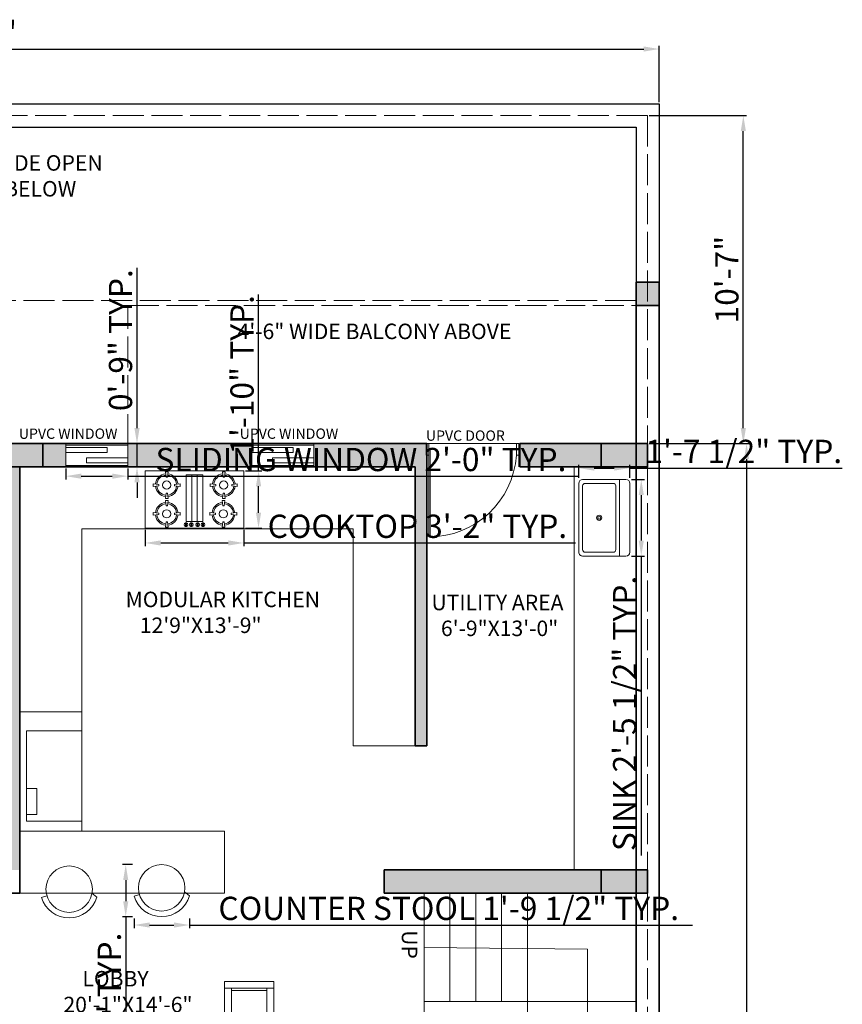
# Model space of a CAD drawing. Units: millimetres. Extents: x 595116 to 630915, y 909473 to 920225.
# Tile 134 of 134: x 630577 to 630895, y 919741 to 920122. Entities that reach past the tile are written whole.
import ezdxf

# ---------------------------------------------------------------- set-up
doc = ezdxf.new("R2010")
doc.units = ezdxf.units.MM
doc.linetypes.add('ACAD_ISO02W100', pattern=[15, 12, -3])
for name, color, linetype, lineweight in [('A-ANNO-SYMB', 7, 'Continuous', 18), ('A-AREA-IDEN', 7, 'Continuous', 20), ('A-EQPM', 8, 'Continuous', 13), ('A-FLOR-BALC', 152, 'Continuous', 18), ('A-FLOR-FIXT', 9, 'Continuous', 18), ('A-FLOR-OVHD', 253, 'ACAD_ISO02W100', 13), ('A-FLOR-STRS-HIDN', 142, 'ACAD_ISO02W100', 13), ('A-FURN', 32, 'Continuous', 18), ('A-WALL', 1, 'Continuous', 35), ('A-WALL-PATT', 8, 'Continuous', 13), ('C-PROP', 7, 'Continuous', 25), ('C-PROP-REF', 240, 'ACAD_ISO02W100', 13), ('Column', 6, 'Continuous', 35), ('Dimension', 3, 'Continuous', 18), ('Doors', 31, 'Continuous', 20), ('STAIR CASE', 142, 'Continuous', 20), ('Text', 7, 'Continuous', 18), ('Windows', 33, 'Continuous', 18)]:
    doc.layers.add(name, color=color, linetype=linetype, lineweight=lineweight)
doc.styles.get("Standard").update_dxf_attribs({"font": 'arial.ttf'})
doc.dimstyles.new('ISO-25', dxfattribs={"dimtxt": 9, "dimasz": 6, "dimexe": 1.25, "dimexo": 0.625, "dimtad": 1, "dimlunit": 4, "dimtxsty": 'Standard', "dimcen": 2.5, "dimadec": 0, "dimazin": 0, "dimtfac": 1, "dimtmove": 0, "dimatfit": 3, "dimfxl": 1, "dimarcsym": 0})

# ---------------------------------------------------------------- blocks, each defined once
blk = doc.blocks.new('KWD')
for points in [[(629753.63, 919957.93), (629752.54, 919957.93), (629752.54, 919953.43), (629753.63, 919953.43)], [(629787.45, 919957.93), (629787.45, 919953.43), (629788.54, 919953.43), (629788.54, 919957.93)]]:
    blk.add_lwpolyline(points, close=True)
blk.add_lwpolyline([(629753.63, 919921.79), (629753.63, 919955.68), (629754.13, 919955.68), (629754.13, 919921.8)])
blk.add_arc((629753.64, 919955.68), 33.88, 269.99, 356.196)
blk = doc.blocks.new('A$C57CF26DA')
for p, q in [((0, 0), (0, 420)), ((720, 420), (0, 420)), ((166.9, 413), (146.9, 413)), ((146.9, 413), (151.9, 373)), ((151.9, 373), (161.9, 373)), ((161.9, 373), (166.9, 413)), ((300, 390.9), (300, 49.1)), ((300, 390.9), (420, 390.9)), ((340, 390.9), (340, 49.1)), ((380, 390.9), (380, 49.1)), ((420, 390.9), (420, 49.1)), ((583.6, 413), (563.6, 413)), ((563.6, 413), (568.6, 373)), ((568.6, 373), (578.6, 373)), ((578.6, 373), (583.6, 413)), ((720, 0), (720, 420)), ((98.9, 320), (58.9, 325)), ((58.9, 325), (58.9, 305)), ((58.9, 305), (98.9, 310)), ((98.9, 310), (98.9, 320)), ((254.8, 325), (214.8, 320)), ((214.8, 320), (214.8, 310)), ((214.8, 310), (254.8, 305)), ((254.8, 305), (254.8, 325)), ((515.6, 320), (475.6, 325)), ((475.6, 325), (475.6, 305)), ((475.6, 305), (515.6, 310)), ((515.6, 310), (515.6, 320)), ((671.6, 325), (631.6, 320)), ((631.6, 320), (631.6, 310)), ((631.6, 310), (671.6, 305)), ((671.6, 305), (671.6, 325)), ((151.9, 257), (146.9, 217)), ((146.9, 217), (166.9, 217)), ((161.9, 257), (151.9, 257)), ((166.9, 217), (161.9, 257)), ((568.6, 257), (563.6, 217)), ((563.6, 217), (583.6, 217)), ((578.6, 257), (568.6, 257)), ((583.6, 217), (578.6, 257)), ((166.9, 203), (146.9, 203)), ((146.9, 203), (151.9, 163)), ((151.9, 163), (161.9, 163)), ((161.9, 163), (166.9, 203)), ((581.1, 203), (561.1, 203)), ((561.1, 203), (566.1, 163)), ((566.1, 163), (576.1, 163)), ((576.1, 163), (581.1, 203)), ((98.9, 110), (58.9, 115)), ((58.9, 115), (58.9, 95)), ((58.9, 95), (98.9, 100)), ((98.9, 100), (98.9, 110)), ((254.8, 115), (214.8, 110)), ((214.8, 110), (214.8, 100)), ((214.8, 100), (254.8, 95)), ((254.8, 95), (254.8, 115)), ((513.1, 110), (473.1, 115)), ((473.1, 115), (473.1, 95)), ((473.1, 95), (513.1, 100)), ((513.1, 100), (513.1, 110)), ((669, 115), (629, 110)), ((629, 110), (629, 100)), ((629, 100), (669, 95)), ((669, 95), (669, 115)), ((151.9, 47), (146.9, 7)), ((146.9, 7), (166.9, 7)), ((161.9, 47), (151.9, 47)), ((166.9, 7), (161.9, 47)), ((301.5, 38.7), (294.7, 38.7)), ((294.7, 38.7), (294.7, 11.3)), ((294.7, 11.3), (301.5, 11.3)), ((420, 49.1), (300, 49.1)), ((301.5, 11.3), (301.5, 38.7)), ((340.5, 38.7), (333.7, 38.7)), ((333.7, 38.7), (333.7, 11.3)), ((333.7, 11.3), (340.5, 11.3)), ((340.5, 11.3), (340.5, 38.7)), ((379.7, 11.3), (379.7, 38.7)), ((379.7, 38.7), (386.5, 38.7)), ((386.5, 11.3), (379.7, 11.3)), ((386.5, 38.7), (386.5, 11.3)), ((418.7, 11.3), (418.7, 38.7)), ((418.7, 38.7), (425.5, 38.7)), ((425.5, 11.3), (418.7, 11.3)), ((425.5, 38.7), (425.5, 11.3)), ((566.1, 47), (561.1, 7)), ((561.1, 7), (581.1, 7)), ((576.1, 47), (566.1, 47)), ((581.1, 7), (576.1, 47)), ((720, 0), (0, 0))]:
    blk.add_line(p, q)
for centre in [(156.9, 315), (573.6, 315), (156.9, 105), (571.1, 105)]:
    blk.add_circle(centre, 30)
for centre, radius, start, end in [((156.9, 315), 83, 95.58493, 174.41507), ((156.9, 315), 73, 95.37384, 174.62616), ((156.9, 315), 73, 5.37384, 84.62616), ((156.9, 315), 83, 5.58493, 84.41507), ((573.6, 315), 83, 95.58493, 174.41507), ((573.6, 315), 73, 95.37384, 174.62616), ((573.6, 315), 73, 5.37384, 84.62616), ((573.6, 315), 83, 5.58493, 84.41507), ((156.9, 315), 83, 185.58493, 264.41507), ((156.9, 315), 73, 185.37384, 264.62616), ((156.9, 315), 73, 275.37384, 354.62616), ((156.9, 315), 83, 275.58493, 354.41507), ((573.6, 315), 83, 185.58493, 264.41507), ((573.6, 315), 73, 185.37384, 264.62616), ((573.6, 315), 73, 275.37384, 354.62616), ((573.6, 315), 83, 275.58493, 354.41507), ((156.9, 105), 83, 95.58493, 174.41507), ((156.9, 105), 73, 95.37384, 174.62616), ((156.9, 105), 73, 5.37384, 84.62616), ((156.9, 105), 83, 5.58493, 84.41507), ((571.1, 105), 83, 95.58493, 174.41507), ((571.1, 105), 73, 95.37384, 174.62616), ((571.1, 105), 73, 5.37384, 84.62616), ((571.1, 105), 83, 5.58493, 84.41507), ((156.9, 105), 83, 185.58493, 264.41507), ((156.9, 105), 73, 185.37384, 264.62616), ((156.9, 105), 73, 275.37384, 354.62616), ((156.9, 105), 83, 275.58493, 354.41507), ((571.1, 105), 83, 185.58493, 264.41507), ((571.1, 105), 73, 185.37384, 264.62616), ((571.1, 105), 73, 275.37384, 354.62616), ((571.1, 105), 83, 275.58493, 354.41507), ((298.1, 25), 13.7, 104.47751, 255.52249), ((298.1, 25), 13.7, 284.47751, 75.52249), ((337.1, 25), 13.7, 104.47751, 255.52249), ((337.1, 25), 13.7, 284.47751, 75.52249), ((383.1, 25), 13.7, 104.47751, 255.52249), ((383.1, 25), 13.7, 284.47751, 75.52249), ((422.1, 25), 13.7, 104.47751, 255.52249), ((422.1, 25), 13.7, 284.47751, 75.52249)]:
    blk.add_arc(centre, radius, start, end)
blk = doc.blocks.new('Sink-single - 30 in top')
blk.add_line((-15, -3.999996), (15, -3.999996))
for points in [[(-13.5, 0), (13.5, 0)], [(-15, -18.499996), (-15, -1.5)], [(15, -1.5), (15, -18.499996)], [(-13.5, -17.499996), (-13.5, -6.499996)], [(-12.5, -5.499996), (12.5, -5.499996)], [(13.5, -6.499996), (13.5, -17.499996)], [(12.5, -18.499996), (-12.5, -18.499996)], [(13.5, -19.999996), (-13.5, -19.999996)]]:
    blk.add_lwpolyline(points)
for radius in [1, 0.5]:
    blk.add_circle((0, -11.999996), radius)
for centre, radius, start, end in [((-13.5, -1.5), 1.5, 90, 180), ((13.5, -1.5), 1.5, 0, 90), ((-12.5, -6.499996), 1, 90, 180), ((12.5, -6.499996), 1, 0, 90), ((-13.5, -18.499996), 1.5, 180, 270), ((-12.5, -17.499996), 1, 180, 270), ((12.5, -17.499996), 1, 270, 0), ((13.5, -18.499996), 1.5, 270, 0)]:
    blk.add_arc(centre, radius, start, end)
blk = doc.blocks.new('DINING')
for p, q in [((630176.61, 919568.69), (630176.61, 919601.05)), ((630176.61, 919601.05), (630208.41, 919601.05)), ((630176.61, 919596.78), (630208.41, 919596.78)), ((630181.05, 919571.76), (630181.05, 919596.78)), ((630203.97, 919571.76), (630203.97, 919596.78)), ((630208.41, 919601.05), (630208.41, 919568.69)), ((630181.05, 919595.21), (630203.97, 919595.21)), ((630163.47, 919568.69), (630222.04, 919568.69)), ((630163.47, 919453.21), (630163.47, 919568.69)), ((630164.11, 919568.05), (630221.39, 919568.05)), ((630164.11, 919453.85), (630164.11, 919568.05)), ((630176.61, 919570.82), (630180.11, 919570.82)), ((630208.41, 919570.82), (630204.91, 919570.82)), ((630221.39, 919568.05), (630221.39, 919453.85)), ((630222.04, 919568.69), (630222.04, 919453.21)), ((630163.47, 919544.57), (630135.12, 919544.57)), ((630135.12, 919544.57), (630135.12, 919519)), ((630137.93, 919544.57), (630137.93, 919519)), ((630138.72, 919544.57), (630138.72, 919519)), ((630222.04, 919544.57), (630250.39, 919544.57)), ((630246.79, 919544.57), (630246.79, 919519)), ((630247.58, 919544.57), (630247.58, 919519)), ((630250.39, 919544.57), (630250.39, 919519)), ((630135.12, 919519), (630163.47, 919519)), ((630250.39, 919519), (630222.04, 919519)), ((630163.47, 919503.52), (630135.12, 919503.52)), ((630135.12, 919503.52), (630135.12, 919477.96)), ((630137.93, 919503.52), (630137.93, 919477.96)), ((630138.72, 919503.52), (630138.72, 919477.96)), ((630222.04, 919503.52), (630250.39, 919503.52)), ((630246.79, 919503.52), (630246.79, 919477.96)), ((630247.58, 919503.52), (630247.58, 919477.96)), ((630250.39, 919503.52), (630250.39, 919477.96)), ((630135.12, 919477.96), (630163.47, 919477.96)), ((630250.39, 919477.96), (630222.04, 919477.96)), ((630222.04, 919453.21), (630163.47, 919453.21)), ((630221.39, 919453.85), (630164.11, 919453.85)), ((630176.61, 919453.21), (630176.61, 919420.86)), ((630176.61, 919451.09), (630180.11, 919451.09)), ((630181.05, 919450.14), (630181.05, 919425.13)), ((630203.97, 919450.14), (630203.97, 919425.13)), ((630208.41, 919451.09), (630204.91, 919451.09)), ((630208.41, 919420.86), (630208.41, 919453.21)), ((630176.61, 919425.13), (630208.41, 919425.13)), ((630181.05, 919426.7), (630203.97, 919426.7)), ((630176.61, 919420.86), (630208.41, 919420.86))]:
    blk.add_line(p, q)
for centre, start, end in [((630180.11, 919571.76), 270, 0), ((630204.91, 919571.76), 180, 270), ((630180.11, 919450.14), 0, 90), ((630204.91, 919450.14), 90, 180)]:
    blk.add_arc(centre, 0.945, start, end)
blk = doc.blocks.new('*D129')
at = {"layer": 'Defpoints', "color": 0, "transparency": 16777216}
for p in [(630824.6, 920110.68), (630293.6, 920089.43), (630824.6, 920089.43)]:
    blk.add_point(p, dxfattribs=at)
at = {"layer": 'Dimension', "color": 0, "lineweight": -2, "transparency": 16777216}
for p, q in [((630293.6, 920090.05), (630293.6, 920111.93)), ((630824.6, 920090.05), (630824.6, 920111.93)), ((630299.6, 920110.68), (630818.6, 920110.68))]:
    blk.add_line(p, q, dxfattribs=at)
at = {"layer": 'Dimension', "color": 0, "transparency": 16777216}
for points in [[(630299.6, 920111.68), (630299.6, 920109.68), (630293.6, 920110.68)], [(630818.6, 920111.68), (630818.6, 920109.68), (630824.6, 920110.68)]]:
    blk.add_solid(points, dxfattribs=at)
at = {"layer": 'Dimension', "color": 0, "transparency": 16777216, "insert": (630559.1, 920115.9), "char_height": 9, "attachment_point": 5}
blk.add_mtext('44\'-3"', dxfattribs=at)
blk = doc.blocks.new('*D130')
at = {"layer": 'Defpoints', "color": 0, "transparency": 16777216}
for p in [(630820.1, 920084.93), (630857.12, 920084.93), (630820.1, 919957.93)]:
    blk.add_point(p, dxfattribs=at)
at = {"layer": 'Dimension', "color": 0, "lineweight": -2, "transparency": 16777216}
for p, q in [((630820.72, 920084.93), (630858.37, 920084.93)), ((630857.12, 919963.93), (630857.12, 920078.93)), ((630820.72, 919957.93), (630858.37, 919957.93))]:
    blk.add_line(p, q, dxfattribs=at)
at = {"layer": 'Dimension', "color": 0, "transparency": 16777216}
for points in [[(630856.12, 920078.93), (630858.12, 920078.93), (630857.12, 920084.93)], [(630856.12, 919963.93), (630858.12, 919963.93), (630857.12, 919957.93)]]:
    blk.add_solid(points, dxfattribs=at)
at = {"layer": 'Dimension', "color": 0, "transparency": 16777216, "insert": (630851.9, 920021.43), "char_height": 9, "attachment_point": 5, "rotation": 90}
blk.add_mtext('10\'-7"', dxfattribs=at)
blk = doc.blocks.new('*D131')
at = {"layer": 'Defpoints', "color": 0, "transparency": 16777216}
for p in [(630820.1, 919957.93), (630820.1, 919360.93), (630858.37, 919360.93)]:
    blk.add_point(p, dxfattribs=at)
at = {"layer": 'Dimension', "color": 0, "lineweight": -2, "transparency": 16777216}
for p, q in [((630820.72, 919957.93), (630859.62, 919957.93)), ((630858.37, 919951.93), (630858.37, 919366.93)), ((630820.72, 919360.93), (630859.62, 919360.93))]:
    blk.add_line(p, q, dxfattribs=at)
at = {"layer": 'Dimension', "color": 0, "transparency": 16777216}
for points in [[(630857.37, 919951.93), (630859.37, 919951.93), (630858.37, 919957.93)], [(630857.37, 919366.93), (630859.37, 919366.93), (630858.37, 919360.93)]]:
    blk.add_solid(points, dxfattribs=at)
at = {"layer": 'Dimension', "color": 0, "transparency": 16777216, "insert": (630853.15, 919659.43), "char_height": 9, "attachment_point": 5, "rotation": 90}
blk.add_mtext('49\'-9"', dxfattribs=at)
blk = doc.blocks.new('WIN-SLIDING-2FT')
for p, q in [((0, 9), (0, 0)), ((0, 9), (24, 9)), ((24, 9), (24, 0)), ((0, 7.5), (16, 7.5)), ((0, 5.5), (16, 5.5)), ((16, 7.5), (16, 5.5)), ((8, 3.5), (24, 3.5)), ((8, 3.5), (8, 1.5)), ((8, 1.5), (24, 1.5)), ((0, 0), (24, 0))]:
    blk.add_line(p, q)
blk.add_lwpolyline([(0, 8.46), (24, 8.46), (24, 0.48), (0, 0.48)], close=True)
blk = doc.blocks.new('WIN-UPVC-2FT')
for p, q in [((0, 9), (0, 0)), ((0, 9), (24, 9)), ((24, 9), (24, 0)), ((0, 7.5), (16, 7.5)), ((0, 0), (24, 0))]:
    blk.add_line(p, q)
blk.add_lwpolyline([(0, 8.46), (24, 8.46), (24, 0.48), (0, 0.48)], close=True)
for points in [[(0, 5.5), (16, 5.5), (16, 7.5)], [(24, 1.5), (8, 1.5), (8, 3.5), (24, 3.5)]]:
    blk.add_lwpolyline(points)
blk = doc.blocks.new('CHAIR-ROUND-2')
for p, q in [((12.11, 21.41), (10.53, 19.55)), ((12.22, 0), (11.59, 2.08))]:
    blk.add_line(p, q)
blk.add_circle((8.99, 10.69), 8.99)
blk.add_arc((8.99, 10.69), 11.16, 286.7943, 73.7898)
blk = doc.blocks.new('KITCHEN-APPLIANCE')
for points in [[(0, 35.07), (21.33, 35.07), (21.33, 0), (0, 0)], [(0, 12.66), (4.02, 12.66), (4.02, 2.57), (0, 2.57)]]:
    blk.add_lwpolyline(points, close=True)
blk = doc.blocks.new('COLUMN-SQUARE-9IN')
h = blk.add_hatch(color=256)
h.dxf.hatch_style = 1
h.paths.add_polyline_path([(9, 9), (0, 9), (0, 0), (9, 0)])
blk.add_lwpolyline([(0, 9), (9, 9), (9, 0), (0, 0)], close=True)
blk = doc.blocks.new('COLUMN-RECT-18X9')
h = blk.add_hatch(color=256)
h.dxf.hatch_style = 1
h.paths.add_polyline_path([(18, 9), (0, 9), (0, 0), (18, 0)])
blk.add_lwpolyline([(0, 9), (18, 9), (18, 0), (0, 0)], close=True)
blk = doc.blocks.new('COLUMN-RECT-18X9-B')
h = blk.add_hatch(color=256)
h.dxf.hatch_style = 1
h.paths.add_polyline_path([(18, 0), (18, 9), (0, 9), (0, 0)])
blk.add_lwpolyline([(0, 9), (18, 9), (18, 0), (0, 0)], close=True)
blk = doc.blocks.new('*D166')
at = {"layer": 'Defpoints', "color": 0, "transparency": 16777216}
for p in [(630813.19, 919944.02), (630813.19, 919914.41), (630817.63, 919914.41)]:
    blk.add_point(p, dxfattribs=at)
at = {"layer": 'Dimension', "color": 0, "lineweight": -2, "transparency": 16777216}
for p, q in [((630813.81, 919944.02), (630818.88, 919944.02)), ((630817.63, 919938.02), (630817.63, 919920.41)), ((630813.81, 919914.41), (630818.88, 919914.41)), ((630817.63, 919914.41), (630817.63, 919798.53))]:
    blk.add_line(p, q, dxfattribs=at)
at = {"layer": 'Dimension', "color": 0, "transparency": 16777216}
for points in [[(630816.63, 919938.02), (630818.63, 919938.02), (630817.63, 919944.02)], [(630816.63, 919920.41), (630818.63, 919920.41), (630817.63, 919914.41)]]:
    blk.add_solid(points, dxfattribs=at)
at = {"layer": 'Dimension', "color": 0, "transparency": 16777216, "insert": (630812.35, 919853.47), "char_height": 9, "attachment_point": 5, "rotation": 90}
blk.add_mtext('SINK 2\'-5 1/2" TYP.', dxfattribs=at)
blk = doc.blocks.new('*D167')
at = {"layer": 'Defpoints', "color": 0, "transparency": 16777216}
for p in [(630813.19, 919948.47), (630793.44, 919944.02), (630813.19, 919944.02)]:
    blk.add_point(p, dxfattribs=at)
at = {"layer": 'Dimension', "color": 0, "lineweight": -2, "transparency": 16777216}
for p, q in [((630793.44, 919944.65), (630793.44, 919949.72)), ((630799.44, 919948.47), (630807.19, 919948.47)), ((630813.19, 919944.65), (630813.19, 919949.72)), ((630813.19, 919948.47), (630895.42, 919948.47))]:
    blk.add_line(p, q, dxfattribs=at)
at = {"layer": 'Dimension', "color": 0, "transparency": 16777216}
for points in [[(630799.44, 919949.47), (630799.44, 919947.47), (630793.44, 919948.47)], [(630807.19, 919949.47), (630807.19, 919947.47), (630813.19, 919948.47)]]:
    blk.add_solid(points, dxfattribs=at)
at = {"layer": 'Dimension', "color": 0, "transparency": 16777216, "insert": (630857.3, 919953.75), "char_height": 9, "attachment_point": 5}
blk.add_mtext('1\'-7 1/2" TYP.', dxfattribs=at)
blk = doc.blocks.new('*D170')
at = {"layer": 'Defpoints', "color": 0, "transparency": 16777216}
for p in [(630621.34, 919774.78), (630642.75, 919774.78), (630642.75, 919771.57)]:
    blk.add_point(p, dxfattribs=at)
at = {"layer": 'Dimension', "color": 0, "lineweight": -2, "transparency": 16777216}
for p, q in [((630621.34, 919774.15), (630621.34, 919770.32)), ((630642.75, 919774.15), (630642.75, 919770.32)), ((630627.34, 919771.57), (630636.75, 919771.57)), ((630642.75, 919771.57), (630837.5, 919771.57))]:
    blk.add_line(p, q, dxfattribs=at)
at = {"layer": 'Dimension', "color": 0, "transparency": 16777216}
for points in [[(630627.34, 919772.57), (630627.34, 919770.57), (630621.34, 919771.57)], [(630636.75, 919772.57), (630636.75, 919770.57), (630642.75, 919771.57)]]:
    blk.add_solid(points, dxfattribs=at)
at = {"layer": 'Dimension', "color": 0, "transparency": 16777216, "insert": (630743.12, 919776.85), "char_height": 9, "attachment_point": 5}
blk.add_mtext('COUNTER STOOL 1\'-9 1/2" TYP.', dxfattribs=at)
blk = doc.blocks.new('*D171')
at = {"layer": 'Defpoints', "color": 0, "transparency": 16777216}
for p in [(630621.34, 919794.96), (630618.13, 919774.78), (630621.34, 919774.78)]:
    blk.add_point(p, dxfattribs=at)
at = {"layer": 'Dimension', "color": 0, "lineweight": -2, "transparency": 16777216}
for p, q in [((630620.72, 919794.96), (630616.88, 919794.96)), ((630618.13, 919788.96), (630618.13, 919780.78)), ((630620.72, 919774.78), (630616.88, 919774.78)), ((630618.13, 919774.78), (630618.13, 919713.52))]:
    blk.add_line(p, q, dxfattribs=at)
at = {"layer": 'Dimension', "color": 0, "transparency": 16777216}
for points in [[(630617.13, 919788.96), (630619.13, 919788.96), (630618.13, 919794.96)], [(630617.13, 919780.78), (630619.13, 919780.78), (630618.13, 919774.78)]]:
    blk.add_solid(points, dxfattribs=at)
at = {"layer": 'Dimension', "color": 0, "transparency": 16777216, "insert": (630612.91, 919741.15), "char_height": 9, "attachment_point": 5, "rotation": 90}
blk.add_mtext('1\'-8" TYP.', dxfattribs=at)
blk = doc.blocks.new('*D184')
at = {"layer": 'Defpoints', "color": 0, "transparency": 16777216}
for p in [(630625.67, 919925.19), (630663.8, 919925.19), (630663.8, 919919.47)]:
    blk.add_point(p, dxfattribs=at)
at = {"layer": 'Dimension', "color": 0, "lineweight": -2, "transparency": 16777216}
for p, q in [((630625.67, 919924.57), (630625.67, 919918.22)), ((630663.8, 919924.57), (630663.8, 919918.22)), ((630631.67, 919919.47), (630657.8, 919919.47)), ((630663.8, 919919.47), (630792.17, 919919.47))]:
    blk.add_line(p, q, dxfattribs=at)
at = {"layer": 'Dimension', "color": 0, "transparency": 16777216}
for points in [[(630631.67, 919920.47), (630631.67, 919918.47), (630625.67, 919919.47)], [(630657.8, 919920.47), (630657.8, 919918.47), (630663.8, 919919.47)]]:
    blk.add_solid(points, dxfattribs=at)
at = {"layer": 'Dimension', "color": 0, "transparency": 16777216, "insert": (630730.99, 919924.76), "char_height": 9, "attachment_point": 5}
blk.add_mtext('COOKTOP 3\'-2" TYP.', dxfattribs=at)
blk = doc.blocks.new('*D185')
at = {"layer": 'Defpoints', "color": 0, "transparency": 16777216}
for p in [(630663.8, 919947.44), (630669.52, 919947.44), (630663.8, 919925.19)]:
    blk.add_point(p, dxfattribs=at)
at = {"layer": 'Dimension', "color": 0, "lineweight": -2, "transparency": 16777216}
for p, q in [((630669.52, 919947.44), (630669.52, 920015.69)), ((630664.43, 919947.44), (630670.77, 919947.44)), ((630669.52, 919931.19), (630669.52, 919941.44)), ((630664.43, 919925.19), (630670.77, 919925.19))]:
    blk.add_line(p, q, dxfattribs=at)
at = {"layer": 'Dimension', "color": 0, "transparency": 16777216}
for points in [[(630668.52, 919941.44), (630670.52, 919941.44), (630669.52, 919947.44)], [(630668.52, 919931.19), (630670.52, 919931.19), (630669.52, 919925.19)]]:
    blk.add_solid(points, dxfattribs=at)
at = {"layer": 'Dimension', "color": 0, "transparency": 16777216, "insert": (630664.3, 919984.56), "char_height": 9, "attachment_point": 5, "rotation": 90}
blk.add_mtext('1\'-10" TYP.', dxfattribs=at)
blk = doc.blocks.new('*D194')
at = {"layer": 'Defpoints', "color": 0, "transparency": 16777216}
for p in [(630594.89, 919948.93), (630618.89, 919948.93), (630618.89, 919945.33)]:
    blk.add_point(p, dxfattribs=at)
at = {"layer": 'Dimension', "color": 0, "lineweight": -2, "transparency": 16777216}
for p, q in [((630594.89, 919948.3), (630594.89, 919944.08)), ((630618.89, 919948.3), (630618.89, 919944.08)), ((630600.89, 919945.33), (630612.89, 919945.33)), ((630618.89, 919945.33), (630793.41, 919945.33))]:
    blk.add_line(p, q, dxfattribs=at)
at = {"layer": 'Dimension', "color": 0, "transparency": 16777216}
for points in [[(630600.89, 919946.33), (630600.89, 919944.33), (630594.89, 919945.33)], [(630612.89, 919946.33), (630612.89, 919944.33), (630618.89, 919945.33)]]:
    blk.add_solid(points, dxfattribs=at)
at = {"layer": 'Dimension', "color": 0, "transparency": 16777216, "insert": (630709.15, 919950.61), "char_height": 9, "attachment_point": 5}
blk.add_mtext('SLIDING WINDOW 2\'-0" TYP.', dxfattribs=at)
blk = doc.blocks.new('*D195')
at = {"layer": 'Defpoints', "color": 0, "transparency": 16777216}
for p in [(630618.89, 919957.93), (630622.49, 919957.93), (630618.89, 919948.93)]:
    blk.add_point(p, dxfattribs=at)
at = {"layer": 'Dimension', "color": 0, "lineweight": -2, "transparency": 16777216}
for p, q in [((630622.49, 919963.93), (630622.49, 920026.04)), ((630619.52, 919957.93), (630623.74, 919957.93)), ((630622.49, 919948.93), (630622.49, 919957.93)), ((630619.52, 919948.93), (630623.74, 919948.93)), ((630622.49, 919942.93), (630622.49, 919936.93))]:
    blk.add_line(p, q, dxfattribs=at)
at = {"layer": 'Dimension', "color": 0, "transparency": 16777216}
for points in [[(630621.49, 919963.93), (630623.49, 919963.93), (630622.49, 919957.93)], [(630621.49, 919942.93), (630623.49, 919942.93), (630622.49, 919948.93)]]:
    blk.add_solid(points, dxfattribs=at)
at = {"layer": 'Dimension', "color": 0, "transparency": 16777216, "insert": (630617.27, 919997.98), "char_height": 9, "attachment_point": 5, "rotation": 90}
blk.add_mtext('0\'-9" TYP.', dxfattribs=at)

msp = doc.modelspace()

# ---------------------------------------------------------------- hatches: boundary and pattern name
at = {"layer": 'A-WALL-PATT'}
h = msp.add_hatch(color=256, dxfattribs=at)
h.dxf.hatch_style = 1
h.paths.add_polyline_path([(630594.891, 919957.928), (630586.096, 919957.928), (630586.096, 919948.928), (630594.891, 919948.928)])
h = msp.add_hatch(color=256, dxfattribs=at)
h.dxf.hatch_style = 1
h.paths.add_polyline_path([(630666.891, 919957.928), (630618.891, 919957.928), (630618.891, 919957.393), (630618.891, 919948.928), (630666.891, 919948.928)])
h = msp.add_hatch(color=256, dxfattribs=at)
h.dxf.hatch_style = 1
h.paths.add_polyline_path([(630734.596, 919957.928), (630690.891, 919957.928), (630690.891, 919948.928), (630730.096, 919948.928), (630730.096, 919840.928), (630734.596, 919840.928)])
h = msp.add_hatch(color=256, dxfattribs=at)
h.dxf.hatch_style = 1
h.paths.add_polyline_path([(630802.096, 919957.928), (630770.391, 919957.928), (630770.391, 919948.928), (630802.096, 919948.928)])
h = msp.add_hatch(color=256, dxfattribs=at)
h.dxf.hatch_style = 1
h.paths.add_polyline_path([(630577.096, 919948.928), (630568.096, 919948.928), (630568.096, 919792.928), (630577.096, 919792.928)])
h = msp.add_hatch(color=256, dxfattribs=at)
h.dxf.hatch_style = 1
h.paths.add_polyline_path([(630802.096, 919792.928), (630718.096, 919792.928), (630718.096, 919783.928), (630802.096, 919783.928)])

# ---------------------------------------------------------------- linework, layer by layer
at = {"layer": 'A-ANNO-SYMB'}
for p, q in [((630733.596, 919762.928), (630796.86, 919762.246)), ((630796.86, 919762.246), (630796.86, 919711.928))]:
    msp.add_line(p, q, dxfattribs=at)
at = {"layer": 'A-FLOR-BALC'}
msp.add_line((630815.596, 920020.393), (630824.596, 920020.393), dxfattribs=at)
at = {"layer": 'A-FLOR-FIXT'}
for p, q in [((630791.596, 919948.928), (630791.596, 919792.928)), ((630601.096, 919924.928), (630706.096, 919924.928)), ((630601.096, 919924.928), (630601.096, 919807.928)), ((630706.096, 919924.928), (630706.096, 919840.928)), ((630577.096, 919854.075), (630601.096, 919854.075)), ((630706.096, 919840.928), (630730.096, 919840.928)), ((630577.096, 919807.928), (630656.319, 919807.928)), ((630656.319, 919807.928), (630656.319, 919783.928)), ((630577.096, 919783.928), (630656.319, 919783.928))]:
    msp.add_line(p, q, dxfattribs=at)
at = {"layer": 'A-FLOR-OVHD'}
for p, q in [((630815.596, 920013.301), (630293.596, 920013.301)), ((630618.891, 919957.393), (630618.891, 920011.393)), ((630618.891, 920011.393), (630824.596, 920011.393))]:
    msp.add_line(p, q, dxfattribs=at)
at = {"layer": 'A-FLOR-STRS-HIDN'}
msp.add_line((630733.596, 919741.928), (630733.596, 919651.928), dxfattribs=at)
at = {"layer": 'A-WALL'}
for p, q in [((630815.596, 920020.393), (630815.596, 919333.928)), ((630298.096, 919957.928), (630734.596, 919957.928)), ((630734.596, 919957.928), (630734.596, 919840.928)), ((630770.391, 919957.928), (630770.391, 919948.928)), ((630770.596, 919957.928), (630770.596, 919948.928)), ((630770.596, 919957.928), (630820.096, 919957.928)), ((630577.096, 919948.928), (630577.096, 919783.928)), ((630577.096, 919948.928), (630730.096, 919948.928)), ((630730.096, 919948.928), (630730.096, 919840.928)), ((630770.596, 919948.928), (630820.096, 919948.928)), ((630730.096, 919840.928), (630734.596, 919840.928)), ((630718.096, 919792.928), (630820.096, 919792.928)), ((630718.096, 919792.928), (630718.096, 919783.928)), ((630508.656, 919783.928), (630577.096, 919783.928)), ((630718.096, 919783.928), (630820.096, 919783.928))]:
    msp.add_line(p, q, dxfattribs=at)
msp.add_lwpolyline([(630824.596, 920020.393), (630824.596, 919333.928)], dxfattribs=at)
at = {"layer": 'C-PROP'}
for p, q in [((630824.596, 920089.428), (630824.596, 920020.393)), ((630302.596, 920080.428), (630815.596, 920080.428)), ((630815.596, 920080.428), (630815.596, 920020.393))]:
    msp.add_line(p, q, dxfattribs=at)
msp.add_lwpolyline([(630293.596, 920089.428), (630824.596, 920089.428)], dxfattribs=at)
at = {"layer": 'C-PROP-REF'}
for p, q in [((630298.096, 920084.928), (630820.096, 920084.928)), ((630820.096, 920084.928), (630820.096, 919150.928))]:
    msp.add_line(p, q, dxfattribs=at)
at = {"layer": 'Doors'}
msp.add_line((630735.484, 919957.928), (630769.298, 919957.928), dxfattribs=at)
at = {"layer": 'STAIR CASE'}
for p, q in [((630733.596, 919783.928), (630733.596, 919741.928)), ((630743.596, 919783.928), (630743.596, 919741.928)), ((630753.596, 919783.928), (630753.596, 919741.928)), ((630763.596, 919783.928), (630763.596, 919741.928)), ((630773.596, 919783.928), (630773.596, 919741.928)), ((630773.596, 919741.928), (630733.596, 919741.928)), ((630773.596, 919741.928), (630815.596, 919741.928)), ((630773.596, 919681.928), (630773.596, 919741.928))]:
    msp.add_line(p, q, dxfattribs=at)
at = {"layer": 'Windows'}
for p, q in [((630594.891, 919957.928), (630594.891, 919948.928)), ((630618.891, 919957.928), (630618.891, 919948.928)), ((630666.891, 919957.928), (630666.891, 919948.928)), ((630690.891, 919957.928), (630690.891, 919948.928))]:
    msp.add_line(p, q, dxfattribs=at)

# ---------------------------------------------------------------- block references
at = {"layer": 'A-EQPM'}
msp.add_blockref('KITCHEN-APPLIANCE', (630579.77, 919811.725), dxfattribs=at)
at = {"layer": 'A-FLOR-FIXT', "xscale": 0.0529604773841383, "yscale": 0.0529604773841383, "zscale": 0.0529604773841383}
msp.add_blockref('A$C57CF26DA', (630625.673, 919925.192), dxfattribs=at)
at = {"layer": 'A-FLOR-FIXT', "xscale": 0.9872623020467125, "yscale": 0.9872623020467125, "zscale": 0.9872623020467125, "rotation": 270}
msp.add_blockref('Sink-single - 30 in top', (630813.185, 919929.215), dxfattribs=at)
at = {"layer": 'A-FURN'}
for p, rotation in [((630621.342, 919794.957), 270.0000000026037), ((630585.524, 919794.46), 270.0000000018366)]:
    msp.add_blockref('CHAIR-ROUND-2', p, dxfattribs=dict(at, rotation=rotation))
at = {"layer": 'A-FURN', "xscale": 0.5984731567659999, "yscale": 0.5984731567659999, "zscale": 0.5984731567659999}
msp.add_blockref('DINING', (253512.563, 369393.149), dxfattribs=at)
at = {"layer": 'Column'}
for name, p in [('COLUMN-SQUARE-9IN', (630815.596, 920011.393)), ('COLUMN-RECT-18X9', (630568.096, 919948.928)), ('COLUMN-RECT-18X9', (630802.096, 919948.928)), ('COLUMN-RECT-18X9-B', (630802.096, 919783.928))]:
    msp.add_blockref(name, p, dxfattribs=at)
at = {"layer": 'Doors'}
msp.add_blockref('KWD', (981.85, 0), dxfattribs=at)
at = {"layer": 'Windows'}
for name, p in [('WIN-SLIDING-2FT', (630594.891, 919948.928)), ('WIN-UPVC-2FT', (630666.891, 919948.928))]:
    msp.add_blockref(name, p, dxfattribs=at)

# ---------------------------------------------------------------- texts
at = {"layer": 'A-ANNO-SYMB', "insert": (630730.964, 919778.734), "char_height": 6, "attachment_point": 1, "rotation": 270}
msp.add_mtext_dynamic_manual_height_columns('{     UP}', width=61.33456, gutter_width=12.5, heights=[0], dxfattribs=at)
at = {"layer": 'A-AREA-IDEN', "char_height": 6, "attachment_point": 1}
for s, width, insert in [('{REAR SIDE OPEN\\P  AREA BELOW}', 125.26422, (630545.614, 920069.59)), ('{   MODULAR KITCHEN\\P      12\'9"X13\'-9"}', 95.74439, (630612.579, 919900.615)), ('{ UTILITY AREA\\P   6\'-9"X13\'-0"}', 83.57324, (630734.596, 919899.428)), ('{      LOBBY\\P  20\'-1"X14\'-6"}', 83.57324, (630590.357, 919753.787))]:
    msp.add_mtext_dynamic_manual_height_columns(s, width=width, gutter_width=12.5, heights=[0], dxfattribs=dict(at, insert=insert))
at = {"layer": 'Text', "attachment_point": 1}
for s, width, insert, char_height in [('{4\'-6" WIDE BALCONY ABOVE}', 118.70658, (630661.407, 920004.377), 6), ('{ UPVC WINDOW}', 61.33456, (630575.546, 919963.779), 4), ('{ UPVC WINDOW}', 61.33456, (630660.997, 919963.779), 4), ('{ UPVC DOOR}', 61.33456, (630733.065, 919963.033), 4)]:
    msp.add_mtext_dynamic_manual_height_columns(s, width=width, gutter_width=12.5, heights=[0], dxfattribs=dict(at, insert=insert, char_height=char_height))

# ---------------------------------------------------------------- dimensions: what is measured, and where the dimension line sits
at = {"layer": 'Dimension'}
dim = msp.add_linear_dim(base=(630824.596, 920110.681), p1=(630293.596, 920089.428), p2=(630824.596, 920089.428), dimstyle='ISO-25', override={"dimclrd": 0, "dimclre": 0, "dimclrt": 0}, dxfattribs=at)
dim.commit()
dim.dimension.update_dxf_attribs({"geometry": '*D129', "text_midpoint": (630559.096, 920115.904)})
for base, p2, picture, middle in [((630857.121, 920084.928), (630820.096, 920084.928), '*D130', (630851.901, 920021.428)), ((630858.371, 919360.928), (630820.096, 919360.928), '*D131', (630853.151, 919659.428))]:
    dim = msp.add_linear_dim(base=base, p1=(630820.096, 919957.928), p2=p2, angle=90, dimstyle='ISO-25', override={"dimclrd": 0, "dimclre": 0, "dimclrt": 0}, dxfattribs=at)
    dim.commit()
    dim.dimension.update_dxf_attribs({"geometry": picture, "text_midpoint": middle})
for base, p1, p2, angle, text, picture, middle in [((630622.491, 919957.928), (630618.891, 919948.928), (630618.891, 919957.928), 90, '<> TYP.', '*D195', (630617.27, 919997.982)), ((630669.524, 919947.436), (630663.804, 919925.192), (630663.804, 919947.436), 90, '<> TYP.', '*D185', (630664.304, 919984.563)), ((630817.628, 919914.406), (630813.185, 919944.024), (630813.185, 919914.406), 270, 'SINK <> TYP.', '*D166', (630812.35, 919853.468)), ((630642.752, 919771.566), (630621.342, 919774.777), (630642.752, 919774.777), 0, 'COUNTER STOOL <> TYP.', '*D170', (630743.125, 919776.848)), ((630618.131, 919774.777), (630621.342, 919794.957), (630621.342, 919774.777), 270, '<> TYP.', '*D171', (630612.911, 919741.146))]:
    dim = msp.add_linear_dim(base=base, p1=p1, p2=p2, angle=angle, text=text, dimstyle='ISO-25', override={"dimdec": 1, "dimlfac": 1, "dimrnd": 0, "dimzin": 1, "dimdsep": 46, "dimlunit": 4, "dimfrac": 2}, dxfattribs=at)
    dim.commit()
    dim.dimension.update_dxf_attribs({"geometry": picture, "text_midpoint": middle})
for base, p1, p2, text, picture, middle in [((630618.891, 919945.328), (630594.891, 919948.928), (630618.891, 919948.928), 'SLIDING WINDOW <> TYP.', '*D194', (630709.152, 919950.609)), ((630813.185, 919948.467), (630793.44, 919944.024), (630813.185, 919944.024), '<> TYP.', '*D167', (630857.302, 919953.745)), ((630663.804, 919919.472), (630625.673, 919925.192), (630663.804, 919925.192), 'COOKTOP <> TYP.', '*D184', (630730.989, 919924.757))]:
    dim = msp.add_linear_dim(base=base, p1=p1, p2=p2, text=text, dimstyle='ISO-25', override={"dimdec": 1, "dimlfac": 1, "dimrnd": 0, "dimzin": 1, "dimdsep": 46, "dimlunit": 4, "dimfrac": 2}, dxfattribs=at)
    dim.commit()
    dim.dimension.update_dxf_attribs({"geometry": picture, "text_midpoint": middle})

doc.saveas('drawing.dxf')
